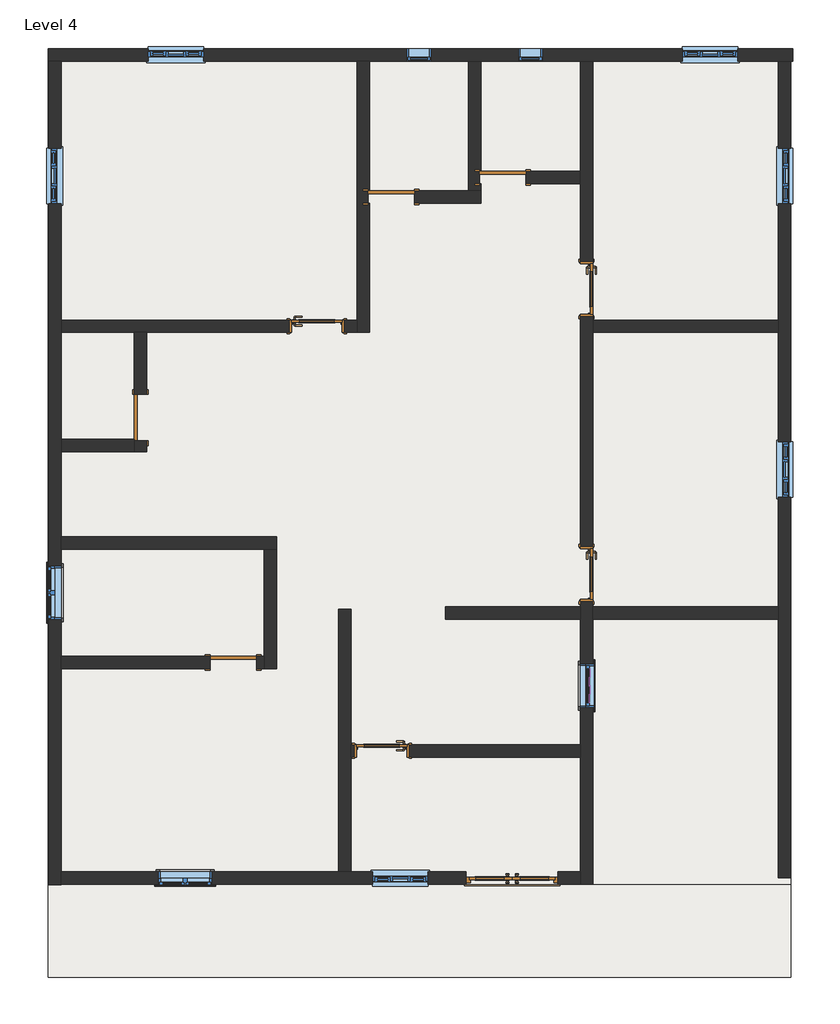
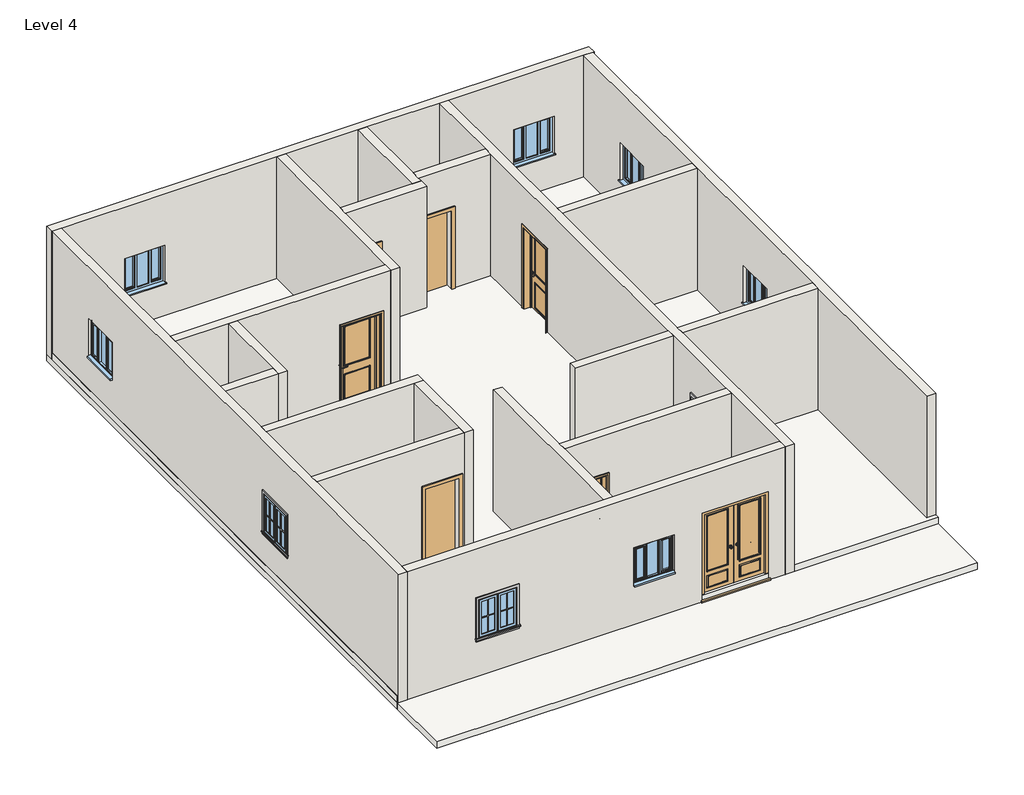
# One storey, incomplete: 19 walls, 12 proxies, 11 windows, 9 doors, 2 slabs, 1 roof.
# Revit data of these elements (continued)
# Element 40 (IfcWall, "9\"") (continued)
#   wall height = 10' - 0"
#   Phase Created = New Construction
#   Base Constraint = Level 4
#   Top Constraint = Level 5
#   Materials on its faces: "Default Wall"
# Elements 41, 42, 43 (IfcWall, "9\" wall")
#   Top Offset = 0' - 0"
#   Base Offset = 0' - 0"
#   wall height = 10' - 0"
#   Phase Created = New Construction
#   Base Constraint = Level 4
#   Top Constraint = Level 5
#   Materials on its faces: "Default Wall"
# Element 44 (IfcWindow, "Fixed : 16\" x 24\"")
#   Mark = "42"
#   Phase Created = New Construction
#   Materials on its faces: "Sash", "Glass"
# Element 45 (IfcWindow, "Fixed : 16\" x 24\"")
#   Mark = "43"
#   Phase Created = New Construction
#   Materials on its faces: "Sash", "Glass"
# Element 46 (IfcWindow, "Window-Casement-Double : 34\" x 36\"")
#   Mark = "34"
#   Window Inset = 0' - 0"
#   Interior Wall Closure = 0' - 2 1/4"
#   Frame Extension = 0' - 0 1/4"
#   Exterior Wall Closure = 0' - 1 1/4"
#   Interior Trim Visibility = yes
#   Exterior Trim Visibility = yes
#   Phase Created = New Construction
#   Materials on its faces: "Wood - Stained", "Glass", "Clad - White"
# Element 47 (IfcWindow, "Window-Casement-Double : 34\" x 36\"")
#   Mark = "35"
#   Window Inset = 0' - 0"
#   Interior Wall Closure = 0' - 2 1/4"
#   Frame Extension = 0' - 0 1/4"
#   Exterior Wall Closure = 0' - 1 1/4"
#   Interior Trim Visibility = yes
#   Exterior Trim Visibility = yes
#   Phase Created = New Construction
#   Materials on its faces: "Wood - Stained", "Glass", "Clad - White"
# Element 48 (IfcWindow, "Window-Double-Hung : 28\" x 46\"")
#   Mark = "44"
#   Window Inset = 0' - 0"
#   Interior Wall Closure = 0' - 1 1/2"
#   Frame Extension = 0' - 1 1/4"
#   Exterior Wall Closure = 0' - 0 1/2"
#   Interior Trim Visibility = yes
#   Indicator Visibility = yes
#   Exterior Trim Visibility = yes
#   Phase Created = New Construction
#   Materials on its faces: "Wood - Stained", "Glass", "Clad - White"
# Element 49 (IfcWindow, "Windows_Tpl_Plain : 910x910mm")
#   Mark = "36"
#   Phase Created = New Construction
#   Materials on its faces: "Window Frame", "Glass"
# Element 50 (IfcWindow, "Windows_Tpl_Plain : 910x910mm")
#   Mark = "39"
#   Phase Created = New Construction
#   Materials on its faces: "Window Frame", "Glass"
# Element 51 (IfcWindow, "Windows_Tpl_Plain : 910x910mm")
#   Mark = "40"
#   Phase Created = New Construction
#   Materials on its faces: "Window Frame", "Glass"
# Element 52 (IfcWindow, "Windows_Tpl_Plain : 910x910mm")
#   Mark = "41"
#   Phase Created = New Construction
#   Materials on its faces: "Window Frame", "Glass"
# Element 53 (IfcWindow, "Windows_Tpl_Plain : 910x910mm")
#   Mark = "37"
#   Phase Created = New Construction
#   Materials on its faces: "Window Frame", "Glass"
# Element 54 (IfcWindow, "Windows_Tpl_Plain : 910x910mm")
#   Mark = "38"
#   Phase Created = New Construction
#   Materials on its faces: "Window Frame", "Glass"
# Materials
#   "Door - Panel": class "Wood", colour RGB 210 159 95, transparency 0, Cost = 0
#   "Door - Glazing": colour RGB 0 0 255, transparency 0.75
#   "Door - Frame/Mullion": class "Wood", colour RGB 212 179 113, transparency 0
#   "Door - Handle": colour RGB 247 247 247, transparency 0
#   "Door - Architrave": class "Wood", colour RGB 154 90 5, transparency 0
#   "Door - Frame": colour RGB 118 70 51, transparency 0, Cost = 0
#   "Glass": class "Glass", colour RGB 0 128 192, transparency 0.75, Description = "Soda Lime Glass", Cost = 0
#   "Sash": class "Wood", colour RGB 224 178 126, transparency 0, Cost = 0
#   "Wood - Stained": class "Wood", colour RGB 224 178 126, transparency 0, Cost = 0
#   "Clad - White": class "Wood", colour RGB 242 242 238, transparency 0, Cost = 0
#   "Window Frame": colour RGB 249 249 249, transparency 0
#   "Default Roof": colour RGB 88 101 114, transparency 0, Cost = 0
#   "Default Floor": colour RGB 128 128 128, transparency 0, Cost = 0
#   "Default Wall": colour RGB 128 128 128, transparency 0, Cost = 0
